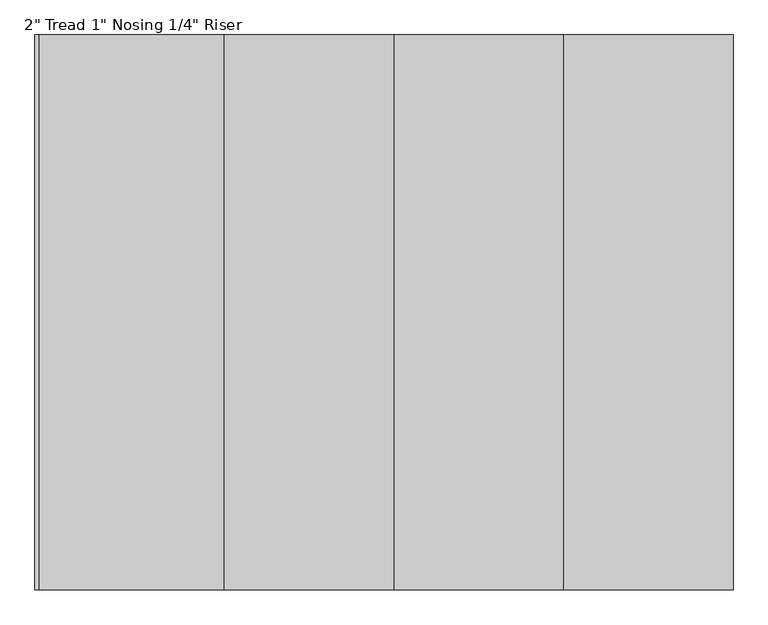
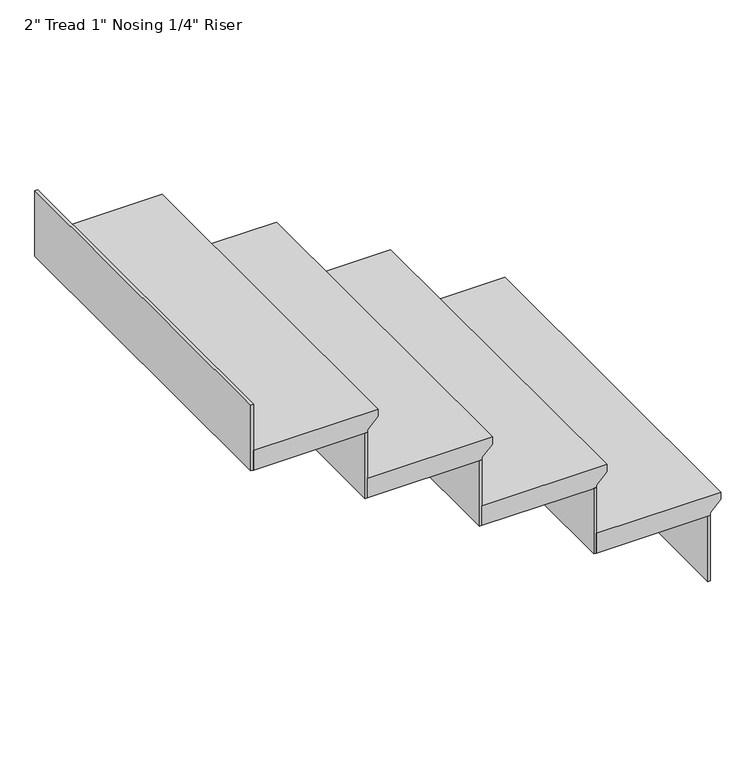
"""IFC4 building model written with IfcOpenShell, lengths in millimetres: stair flight geometry."""

from ifc_helpers import new_model, si_unit, frame, origin, place, context, project, spatial, polyline, outline, extrude, source, transform, mapped, element, save


def stair_flight_c4ab4097(model_context):
    return source(origin(), model_context, "Body", "SweptSolid", [
        extrude(outline(polyline([(2540.0, -7733.3118598), (2540.0, -8038.1118598), (2489.2, -8038.1118598), (2489.2, -7758.7118598), (2495.55, -7758.7118598), (2520.95, -7733.3118598), (2540.0, -7733.3118598)])), frame((0.0, 1647.7368529, 0.0), z_axis=(0.0, 1.0, 0.0), x_axis=(0.0, 0.0, 1.0)), (0.0, 0.0, 1.0), 914.4),
        extrude(outline(polyline([(-7765.0618598, 2562.1368529), (-7758.7118598, 2562.1368529), (-7758.7118598, 1647.7368529), (-7765.0618598, 1647.7368529), (-7765.0618598, 2562.1368529)])), frame((0.0, 0.0, 2319.8666667), z_axis=(0.0, 0.0, 1.0), x_axis=(1.0, 0.0, 0.0)), (0.0, 0.0, 1.0), 169.3333333),
        extrude(outline(polyline([(-8044.4618598, 2562.1368529), (-8038.1118598, 2562.1368529), (-8038.1118598, 1647.7368529), (-8044.4618598, 1647.7368529), (-8044.4618598, 2562.1368529)])), frame((0.0, 0.0, 2489.2), z_axis=(0.0, 0.0, 1.0), x_axis=(1.0, 0.0, 0.0)), (0.0, 0.0, 1.0), 169.3333333),
        extrude(outline(polyline([(2709.3333333, -8012.7118598), (2709.3333333, -8317.5118598), (2658.5333333, -8317.5118598), (2658.5333333, -8038.1118598), (2664.8833333, -8038.1118598), (2690.2833333, -8012.7118598), (2709.3333333, -8012.7118598)])), frame((0.0, 1647.7368529, 0.0), z_axis=(0.0, 1.0, 0.0), x_axis=(0.0, 0.0, 1.0)), (0.0, 0.0, 1.0), 914.4),
        extrude(outline(polyline([(-8323.8618598, 2562.1368529), (-8317.5118598, 2562.1368529), (-8317.5118598, 1647.7368529), (-8323.8618598, 1647.7368529), (-8323.8618598, 2562.1368529)])), frame((0.0, 0.0, 2658.5333333), z_axis=(0.0, 0.0, 1.0), x_axis=(1.0, 0.0, 0.0)), (0.0, 0.0, 1.0), 169.3333333),
        extrude(outline(polyline([(2878.6666667, -8292.1118598), (2878.6666667, -8596.9118598), (2827.8666667, -8596.9118598), (2827.8666667, -8317.5118598), (2834.2166667, -8317.5118598), (2859.6166667, -8292.1118598), (2878.6666667, -8292.1118598)])), frame((0.0, 1647.7368529, 0.0), z_axis=(0.0, 1.0, 0.0), x_axis=(0.0, 0.0, 1.0)), (0.0, 0.0, 1.0), 914.4),
        extrude(outline(polyline([(-8603.2618598, 2562.1368529), (-8596.9118598, 2562.1368529), (-8596.9118598, 1647.7368529), (-8603.2618598, 1647.7368529), (-8603.2618598, 2562.1368529)])), frame((0.0, 0.0, 2827.8666667), z_axis=(0.0, 0.0, 1.0), x_axis=(1.0, 0.0, 0.0)), (0.0, 0.0, 1.0), 169.3333333),
        extrude(outline(polyline([(-8882.6618598, 2562.1368529), (-8876.3118598, 2562.1368529), (-8876.3118598, 1647.7368529), (-8882.6618598, 1647.7368529), (-8882.6618598, 2562.1368529)])), frame((0.0, 0.0, 2997.2), z_axis=(0.0, 0.0, 1.0), x_axis=(1.0, 0.0, 0.0)), (0.0, 0.0, 1.0), 169.3333333),
        extrude(outline(polyline([(3048.0, -8571.5118598), (3048.0, -8876.3118598), (2997.2, -8876.3118598), (2997.2, -8596.9118598), (3003.55, -8596.9118598), (3028.95, -8571.5118598), (3048.0, -8571.5118598)])), frame((0.0, 1647.7368529, 0.0), z_axis=(0.0, 1.0, 0.0), x_axis=(0.0, 0.0, 1.0)), (0.0, 0.0, 1.0), 914.4),
    ])


if __name__ == "__main__":
    model = new_model("IFC4")
    model_context = context("Model", 3, world=origin())
    ifc_project = project(units=[si_unit("LENGTHUNIT", "METRE", prefix="MILLI")], contexts=[model_context])
    site = spatial("IfcSite", under=ifc_project)
    building = spatial("IfcBuilding", under=site)
    placement = place(None, origin())
    stair_flight_shape = stair_flight_c4ab4097(model_context)
    element("IfcStairFlight", 1, ObjectType="2\" Tread 1\" Nosing 1/4\" Riser", at=placement, inside=building, context=model_context, shape_type="MappedRepresentation", body=[
        mapped(stair_flight_shape, transform((0.0, 0.0, 0.0), x_axis=(1.0, 0.0, 0.0), y_axis=(0.0, 1.0, 0.0), z_axis=(0.0, 0.0, 1.0))),
    ])
    save(model, "model.ifc")
